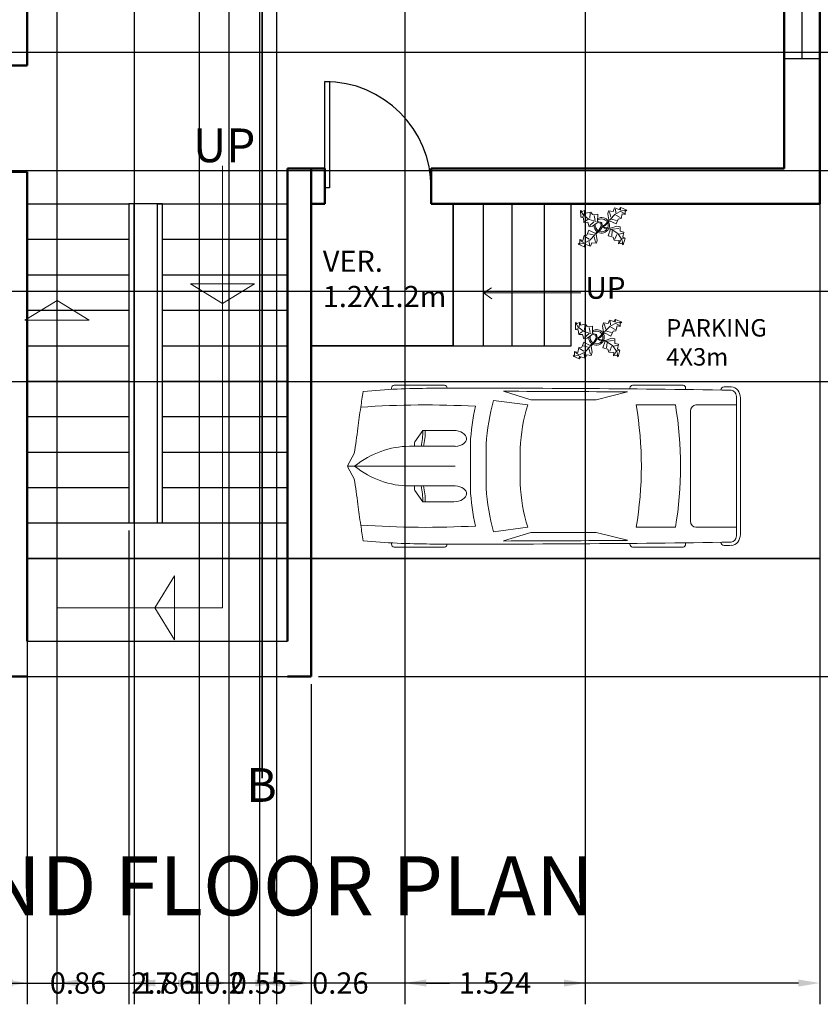
# Model space of a CAD drawing. Units: metres. Extents: x 2443.7 to 2482.9, y 2261.4 to 2287.
# Tile 2 of 8: x 2451.1 to 2457.9, y 2261.4 to 2269.7. Entities that reach past the tile are written whole.
import ezdxf

# ---------------------------------------------------------------- set-up
doc = ezdxf.new("R2010")
doc.units = ezdxf.units.M
doc.linetypes.add('ACAD_ISO02W100', pattern=[15, 12, -3])
for name, color, linetype, lineweight in [('A-ANNO-DIMS', 2, 'Continuous', 18), ('A-ANNO-SYMB', 1, 'Continuous', 18), ('A-AREA-IDEN', 11, 'Continuous', 25), ('A-FLOR-PROJ', 7, 'ACAD_ISO02W100', 18), ('A-MODL', 7, 'Continuous', 25), ('A-WALL', 7, 'Continuous', 50), ('car', 150, 'Continuous', 18), ('door', 6, 'Continuous', 25), ('floor', 7, 'Continuous', 35), ('flower', 70, 'Continuous', 18), ('section', 1, 'Continuous', 35), ('stair', 2, 'Continuous', 25), ('text', 11, 'Continuous', 25), ('window', 3, 'Continuous', 25)]:
    doc.layers.add(name, color=color, linetype=linetype, lineweight=lineweight)
doc.styles.get("Standard").update_dxf_attribs({"font": 'arial.ttf'})
doc.dimstyles.get("Standard").update_dxf_attribs({"dimtxt": 0.18, "dimasz": 0.18, "dimexe": 0.18, "dimexo": 0.0625, "dimgap": 0.09, "dimtad": 0, "dimtih": 1, "dimtoh": 1, "dimdec": 4, "dimzin": 0, "dimdsep": 46, "dimtxsty": 'Standard', "dimcen": 0.09, "dimadec": 0, "dimazin": 0, "dimtfac": 1, "dimtdec": 4, "dimtofl": 0, "dimtmove": 0, "dimatfit": 3, "dimfxl": 1, "dimtolj": 1, "dimtzin": 0, "dimarcsym": 0})

# ---------------------------------------------------------------- blocks, each defined once
blk = doc.blocks.new('*U21')
for p, q in [((0, 0), (0, -6)), ((40, 0), (40, -6))]:
    blk.add_line(p, q)
blk.add_lwpolyline([(0, 0), (0, 40), (1.75, 40), (1.75, 0)], close=True)
blk.add_arc((0, 0), 40, 0, 90)
blk = doc.blocks.new('*U2')
for p, q in [((0, 0), (0, -6)), ((-40, 0), (-40, -6))]:
    blk.add_line(p, q)
blk.add_lwpolyline([(0, 0), (0, 40), (-1.75, 40), (-1.75, 0)], close=True)
blk.add_arc((0, 0), 40, 90, 180)
blk = doc.blocks.new('Plant - Rubber or Philodendron')
for p, q in [((-16.2005, 11.4774), (-13.9899, 8.1064)), ((-16.2005, 11.4774), (-14.8639, 10.7964)), ((-16.0159, 6.3329), (-16.2005, 11.4774)), ((-14.8639, 10.7964), (-12.6195, 11.8975)), ((-13.9899, 8.1064), (-9.5434, 4.7185)), ((-13.3174, 8.325), (-13.0735, 11.0065)), ((-12.6195, 11.8975), (-12.1909, 9.4345)), ((-12.1909, 9.4345), (-8.3829, 10.3)), ((-8.8369, 9.409), (-9.0894, 5.6095)), ((-8.3829, 10.3), (-7.0549, 8.501)), ((-7.0549, 8.501), (-3.0284, 8.6941)), ((-4.8529, 4.012), (-5.7184, 7.82)), ((-3.0284, 8.6941), (-3.0709, 3.1041)), ((4.6914, 8.8812), (5.3859, 11.2828)), ((4.6914, 8.8812), (5.5014, 4.4831)), ((5.3859, 11.2828), (8.8871, 10.7908)), ((5.9878, 10.4842), (7.1971, 6.3869)), ((10.3916, 8.7942), (6.2847, 4.4028)), ((8.8871, 10.7908), (9.9809, 13.4933)), ((9.9809, 13.4933), (13.3837, 12.301)), ((15.3859, 11.3055), (10.3916, 8.7942)), ((10.5828, 12.6946), (10.8893, 9.7953)), ((14.2977, 6.1031), (10.9934, 7.9956)), ((13.3837, 12.301), (14.68, 13.9039)), ((14.5816, 13.2037), (14.3848, 11.8033)), ((14.68, 13.9039), (19.3848, 11.8146)), ((15.7909, 9.1065), (14.8995, 5.3044)), ((15.2875, 10.6053), (17.5907, 9.2105)), ((19.3848, 11.8146), (15.3859, 11.3055)), ((18.1925, 8.4119), (15.7909, 9.1065)), ((19.3848, 11.8146), (18.1868, 10.9119)), ((18.1868, 10.9119), (18.1925, 8.4119)), ((-14.0069, 5.8704), (-16.0159, 6.3329)), ((-15.3434, 6.5514), (-13.9984, 6.9884)), ((-13.5868, 2.2894), (-14.0069, 5.8704)), ((-10.6784, 2.491), (-13.5868, 2.2894)), ((-13.1329, 3.1804), (-10.6614, 4.727)), ((-9.5858, -0.8715), (-10.6784, 2.491)), ((-9.5434, 4.7185), (-4.1917, 2.9888)), ((-9.1318, 0.0195), (-5.9793, 2.9025)), ((-7.1228, -0.443), (-3.5248, 2.2131)), ((-3.5248, 2.2131), (-3.3011, 2.4355)), ((-3.3011, 2.4355), (-0.5306, 1.7947)), ((-3.0709, 3.1041), (0.0797, 2.3163)), ((-0.5306, 1.7947), (-0.2255, -0.5527)), ((-0.5306, 1.7947), (-0.5306, 1.7947)), ((0.0797, 2.3163), (0.4866, -0.031)), ((0.4866, -0.031), (2.1141, 0.2298)), ((2.1141, 0.2298), (5.4346, 3.9146)), ((6.1032, 3.6844), (2.8262, -0.031)), ((5.4346, 3.9146), (5.5014, 4.4831)), ((11.1089, 1.1958), (6.1032, 3.6844)), ((7.7005, 4.8881), (11.5025, 3.9967)), ((12.7005, 4.8994), (11.1089, 1.1958)), ((14.8995, 5.3044), (12.7005, 4.8994)), ((-13.5228, -7.6679), (-11.3237, -7.2629)), ((-11.3237, -7.2629), (-9.7321, -3.5593)), ((-6.3237, -7.2516), (-10.1257, -6.3602)), ((-9.7321, -3.5593), (-4.7264, -6.0479)), ((-7.1228, -0.443), (-9.5858, -0.8715)), ((-9.0148, -11.1577), (-4.9047, -6.8122)), ((-2.019, -3.6148), (-4.7264, -6.0479)), ((-4.1246, -6.8466), (-4.0579, -6.2781)), ((-3.3146, -11.2447), (-4.1246, -6.8466)), ((-4.0579, -6.2781), (-0.9375, -3.1608)), ((-2.019, -3.6148), (-0.2255, -0.5527)), ((-0.9375, -3.1608), (0.5883, -0.8135)), ((0.5883, -0.8135), (2.2447, -2.0916)), ((2.8262, -0.031), (1.3003, -0.5527)), ((1.3003, -0.5527), (2.4193, -1.4655)), ((2.2447, -2.0916), (6.7108, -2.6626)), ((2.4193, -1.4655), (6.895, -2.1175)), ((4.943, -7.9659), (6.7108, -2.6626)), ((11.6605, -0.5413), (6.895, -2.1175)), ((12.3677, -6.1981), (7.219, -2.6772)), ((8.125, -4.0768), (7.7715, -7.9659)), ((8.3544, -2.7453), (13.1973, -2.1704)), ((10.2463, -10.4408), (11.6605, -6.9053)), ((11.6605, -0.5413), (14.1354, -0.8948)), ((15.5496, -10.7943), (12.3677, -6.1981)), ((16.2567, -5.8446), (13.4283, -6.5517)), ((14.1354, -0.8948), (14.1354, -4.4304)), ((14.1354, -4.4304), (16.9638, -5.1375)), ((16.9638, -5.1375), (16.2567, -8.673)), ((-18.008, -14.1781), (-16.8101, -13.2754)), ((-18.008, -14.1781), (-14.0091, -13.669)), ((-13.3032, -16.2674), (-18.008, -14.1781)), ((-16.8157, -10.7754), (-14.4141, -11.4699)), ((-16.8101, -13.2754), (-16.8157, -10.7754)), ((-13.9107, -12.9688), (-16.2139, -11.574)), ((-14.4141, -11.4699), (-13.5228, -7.6679)), ((-14.0091, -13.669), (-9.0148, -11.1577)), ((-12.0069, -14.6645), (-13.3032, -16.2674)), ((-13.2048, -15.5672), (-13.008, -14.1668)), ((-12.921, -8.4665), (-9.6166, -10.359)), ((-8.6042, -15.8568), (-12.0069, -14.6645)), ((-9.206, -15.0581), (-9.5126, -12.1588)), ((-7.5103, -13.1543), (-8.6042, -15.8568)), ((-4.0092, -13.6463), (-7.5103, -13.1543)), ((-4.611, -12.8477), (-5.8203, -8.7504)), ((-3.3146, -11.2447), (-4.0092, -13.6463)), ((8.8321, -9.0266), (4.943, -7.9659)), ((9.5392, -11.1479), (8.8321, -9.0266)), ((13.4283, -11.5015), (9.5392, -11.1479)), ((13.0748, -13.9763), (13.4283, -11.5015)), ((15.5496, -13.6228), (13.0748, -13.9763)), ((14.8425, -10.7943), (13.7819, -13.2692)), ((16.6103, -14.6834), (15.5496, -10.7943)), ((16.6103, -14.6834), (15.5496, -13.6228)), ((17.3174, -9.7337), (15.9032, -9.7337)), ((16.2567, -8.673), (18.0245, -9.7337)), ((18.0245, -9.7337), (16.6103, -14.6834))]:
    blk.add_line(p, q)
for centre, radius, start, end in [((0.0308, 0.1664), 6, 178.6147, 235.1169), ((0.0308, 0.1664), 5, 168.1647, 238.6725), ((0, 0), 6.1275, 34.37569, 120.1028), ((-0.0601, -0.2075), 5.2461, 33.82192, 124.9414), ((-0.2664, 0.1682), 5.2775, 338.4094, 20.03007), ((-0.098, 0.1364), 6.1288, 341.2017, 26.09184), ((-0.0234, 0.3825), 6.1492, 242.5812, 331.2714), ((-0.1102, 0.4886), 5.2883, 247.3711, 327.472)]:
    blk.add_arc(centre, radius, start, end)
blk = doc.blocks.new('*U17')
for p, q in [((46.55, 38.89), (22.35, 38.89)), ((136.7, 38.89), (160.9, 38.89)), ((21.1, 37.41), (21.1, 36.83)), ((47.8, 37.39), (47.8, 37.41)), ((87.99, 31.87), (74.76, 35.92)), ((134.31, 35.6), (119.29, 31.78)), ((135.45, 37.07), (135.45, 37.41)), ((162.15, 37.41), (162.15, 36.77)), ((186.47, -33.5), (186.47, 33.5)), ((70.03, 31.54), (86.41, 29.35)), ((138.42, 29.35), (157.25, 29.35)), ((186.47, 29.35), (167.01, 29.35)), ((188.4, -32.76), (188.4, 32.76)), ((164.52, 26.39), (164.52, -26.39)), ((32.27, 11.63), (36.13, 17.17)), ((36.13, 17.17), (50.94, 17.17)), ((29.77, 9.51), (51.68, 9.51)), ((32.12, 9.51), (32.12, 11.15)), ((58.92, -10.77), (58.92, 10.77)), ((66.55, -10.53), (66.55, 10.53)), ((186.47, -10.53), (186.47, 10.53)), ((3.27, 6.13), (0.1, 0.41)), ((82.74, 8.5), (82.74, -8.5)), ((0, 0), (51.68, 0)), ((0.1, -0.41), (3.27, -6.13)), ((29.77, -9.51), (51.68, -9.51)), ((32.12, -9.51), (32.12, -11.15)), ((32.27, -11.63), (36.13, -17.17)), ((36.13, -17.17), (50.94, -17.17)), ((86.41, -29.35), (70.03, -31.54)), ((87.99, -31.87), (74.76, -35.92)), ((134.31, -35.6), (119.29, -31.78)), ((157.25, -29.35), (138.42, -29.35)), ((167.01, -29.35), (186.47, -29.35)), ((21.1, -37.41), (21.1, -36.83)), ((47.8, -37.39), (47.8, -37.41)), ((135.45, -37.07), (135.45, -37.41)), ((162.15, -37.41), (162.15, -36.77)), ((46.55, -38.89), (22.35, -38.89)), ((136.7, -38.89), (160.9, -38.89))]:
    blk.add_line(p, q)
for centre, major_axis, ratio, start_param, end_param in [((22.35, 37.41), (0, -1.48), 0.842304, 3.141593, 4.712389), ((46.55, 37.41), (0, 1.48), 0.842304, -1.570796, 0), ((136.7, 37.41), (0, -1.48), 0.842304, 3.141593, 4.712389), ((160.9, 37.41), (0, 1.48), 0.842304, -1.570796, 0), ((180.63, 35.84), (0, 2.22), 0.842304, -0.013017, 1.249894), ((64.48, -10556.36), (0, 10595.31), 0.842304, -0.013397, -0.013017), ((183.98, 32.76), (0, -5.25), 0.842304, 1.570796, 3.128196), ((266.03, -27.52), (0, 313.31), 0.842304, 1.367076, 1.39176), ((41.19, -490.86), (0, 528.23), 0.842304, 0.00281, 0.075598), ((64.48, -10555.62), (0, 10593.03), 0.842304, -0.013397, 0.002797), ((64.48, -10555.62), (0, -10591.55), 0.842304, 3.133765, 3.140441), ((183.98, 33.5), (0, -2.96), 0.842304, 1.570796, 3.128196), ((37.47, -593.96), (0, -623.33), 0.842304, 3.096046, 3.200911), ((134.4, 5.39), (0, -89.78), 0.842304, 4.449482, 4.652344), ((135.29, 5.39), (0, 81.77), 0.842304, 1.245306, 1.50788), ((149.6, 2.8), (0, -79.58), 0.842304, 4.372215, 4.640744), ((95.79, -3666.35), (0, -3698.24), 0.842304, 3.134049, 3.144098), ((17.08, 0), (0, 147.02), 0.842304, 4.511394, 4.913384), ((35.91, 0), (0, 147.02), 0.842304, 4.511394, 4.913384), ((167.01, 26.39), (0, 2.96), 0.842304, 0, 1.570796), ((259.18, -27.52), (0, -305.3), 0.842304, 4.528606, 4.561838), ((-204.49, 52.4), (0, -250.96), 0.842304, 1.385369, 1.434372), ((13.04, 17.01), (0, 27.42), 0.842304, 4.435146, 4.718221), ((14.2, 17.01), (0, 27.42), 0.842304, 4.435146, 4.718221), ((50.79, 13.34), (6.34, -0.36), 0.603834, -1.395552, 1.581315), ((29.77, -46.66), (0, 56.17), 0.842304, 0, 0.590319), ((32.75, 11.15), (0, 0.74), 0.842304, 0.879714, 1.570796), ((0.62, 0), (0, -0.74), 0.842304, 4.131459, 5.293319), ((29.77, 46.66), (0, 56.17), 0.842304, 2.551274, 3.141593), ((-204.49, -52.4), (0, 250.96), 0.842304, -1.434372, -1.385369), ((149.6, -2.8), (0, -79.58), 0.842304, -1.499151, -1.230623), ((32.75, -11.15), (0, -0.74), 0.842304, 4.712389, 5.403472), ((13.04, -17.01), (0, -27.42), 0.842304, 1.564964, 1.848039), ((14.2, -17.01), (0, -27.42), 0.842304, 1.564964, 1.848039), ((134.4, -5.39), (0, -89.78), 0.842304, -1.510751, -1.307889), ((135.29, -5.39), (0, -81.77), 0.842304, -1.50788, -1.245306), ((259.18, 27.52), (0, 305.3), 0.842304, 1.721348, 1.754579), ((266.03, 27.52), (0, 313.31), 0.842304, 1.749832, 1.774517), ((37.47, 593.96), (0, -623.33), 0.842304, -0.059319, 0.045547), ((167.01, -26.39), (0, -2.96), 0.842304, 4.712389, 6.283185), ((95.79, 3666.35), (0, -3698.24), 0.842304, -0.002505, 0.007544), ((183.98, -32.76), (0, -5.25), 0.842304, 0.013397, 1.570796), ((41.19, 490.86), (0, -528.23), 0.842304, -0.075598, -0.00281), ((22.35, -37.41), (0, 1.48), 0.842304, 1.570796, 3.141593), ((64.48, 10555.62), (0, 10593.03), 0.842304, 3.138796, 3.15499), ((46.55, -37.41), (0, -1.48), 0.842304, 0, 1.570796), ((64.48, 10555.62), (0, -10591.55), 0.842304, 0.001152, 0.007828), ((136.7, -37.41), (0, -1.48), 0.842304, -1.570796, 0), ((160.9, -37.41), (0, 1.48), 0.842304, 3.141593, 4.712389), ((180.63, -35.84), (0, -2.22), 0.842304, -1.249894, 0.013017), ((183.98, -33.5), (0, 2.96), 0.842304, 3.15499, 4.712389), ((64.48, 10556.36), (0, 10595.31), 0.842304, 3.15461, 3.15499)]:
    blk.add_ellipse(centre, major_axis=major_axis, ratio=ratio, start_param=start_param, end_param=end_param)
at = {"extrusion": (0, 0, -1)}
blk.add_ellipse((50.79, -13.34), major_axis=(6.34, 0.36), ratio=0.603834, start_param=-1.395552, end_param=1.581315, dxfattribs=at)
blk = doc.blocks.new('aditya')
at = {"layer": 'A-ANNO-SYMB'}
for p, q in [((5.15, 3.6226), (5.15, -0.1171)), ((3.752, -0.1171), (3.752, 3.3)), ((5.4209, 2.6227), (4.8791, 2.6227)), ((4.8791, 2.6227), (5.15, 2.4567)), ((5.4209, 2.6227), (5.15, 2.4567)), ((7.3585, 2.5465), (7.4248, 2.5908)), ((8.1818, 2.5465), (7.3585, 2.5465)), ((7.3585, 2.5465), (7.4267, 2.4975)), ((3.481, 2.316), (3.752, 2.4819)), ((4.0229, 2.316), (3.752, 2.4819)), ((3.481, 2.316), (4.0229, 2.316)), ((4.7446, 0.1538), (4.5786, -0.1171)), ((4.7446, -0.388), (4.7446, 0.1538)), ((5.15, -0.1171), (3.752, -0.1171)), ((4.7446, -0.388), (4.5786, -0.1171))]:
    blk.add_line(p, q, dxfattribs=at)
at = {"layer": 'A-FLOR-PROJ', "ltscale": 0.01}
blk.add_line((10.2, 3.3), (10.2, 0.3), dxfattribs=at)
at = {"layer": 'A-WALL'}
for p, q in [((10.2, 3.3), (10.2, 9.9)), ((3.5, 4.4718), (3.5, 5.1521)), ((9.9, 4.8), (9.9, 5)), ((9.9, 3.6), (9.9, 4.8)), ((5.7, -0.4), (5.7, 3.6)), ((5.9, 3.6), (5.7, 3.6)), ((5.9, -0.7), (5.9, 3.6)), ((5.9, 3.6), (6.0153, 3.6)), ((6.9153, 3.6), (9.9, 3.6)), ((3.5, -0.4), (3.5, 3.5718)), ((5.9, 3.3), (6.0153, 3.3)), ((6.9153, 3.3), (10.2, 3.3)), ((3.5, -0.7), (3.2, -0.7)), ((5.7, -0.7), (5.9, -0.7))]:
    blk.add_line(p, q, dxfattribs=at)
for points in [[(3.3, 4.4718), (3.5, 4.4718)], [(6.0153, 3.3), (6.0153, 3.6)], [(6.9153, 3.6), (6.9153, 3.3)], [(3.5, 3.5718), (3.3, 3.5718), (3.3, 3.5742)]]:
    blk.add_lwpolyline(points, dxfattribs=at)
at = {"layer": 'floor'}
for p, q in [((3.5, 0.3), (5.7, 0.3)), ((5.7, 0.3), (9.9, 0.3)), ((10.2, 0.3), (9.9, 0.3))]:
    blk.add_line(p, q, dxfattribs=at)
blk.add_lwpolyline([(6.9153, 3.3), (7.1, 3.3), (7.1, 2.1), (5.9, 2.1), (5.9, 3.3), (6.0153, 3.3)], dxfattribs=at)
at = {"layer": 'section'}
blk.add_line((5.4866, -1.5581), (5.4866, 11.3875), dxfattribs=at)
at = {"layer": 'stair'}
for p, q in [((3.5, 3.3), (4.3595, 3.3)), ((4.6, 3.3), (5.7, 3.3)), ((7.3585, 2.1), (7.3585, 3.3)), ((7.6, 2.1), (7.6, 3.3)), ((7.873, 2.1), (7.873, 3.3)), ((8.1, 2.1), (8.1, 3.3)), ((3.5, 3), (4.3595, 3)), ((4.6423, 3), (5.7, 3)), ((3.5, 2.7), (4.3595, 2.7)), ((4.6423, 2.7), (5.7, 2.7)), ((3.5, 2.4), (4.3595, 2.4)), ((4.6423, 2.4), (5.7, 2.4)), ((3.5, 2.1), (4.3595, 2.1)), ((4.6423, 2.1), (5.7, 2.1)), ((7.1, 2.1), (8.1, 2.1)), ((3.5, 1.8), (4.3595, 1.8)), ((4.6423, 1.8), (5.7, 1.8)), ((3.5, 1.5), (4.3595, 1.5)), ((4.6423, 1.5), (5.7, 1.5)), ((3.5, 1.2), (4.3595, 1.2)), ((4.6423, 1.2), (5.7, 1.2)), ((3.5, 0.9), (4.3595, 0.9)), ((4.6423, 0.9), (5.7, 0.9)), ((3.5, 0.6), (5.7, 0.6)), ((3.5, 0.3), (5.7, 0.3)), ((3.5, -0.4), (5.7, -0.4)), ((3.5, -0.7), (5.7, -0.7))]:
    blk.add_line(p, q, dxfattribs=at)
for points in [[(4.6423, 3.3002), (4.3595, 3.3002), (4.3595, 0.6), (4.6423, 0.6)], [(4.6008, 3.3002), (4.4009, 3.3002), (4.4001, 0.6), (4.6, 0.6)]]:
    blk.add_lwpolyline(points, close=True, dxfattribs=at)
at = {"layer": 'window'}
blk.add_line((10.05, 5.7272), (10.05, 4.5272), dxfattribs=at)
blk.add_lwpolyline([(9.9, 5.7272), (10.2, 5.7272), (10.2, 4.5272), (9.9, 4.5272)], close=True, dxfattribs=at)
at = {"layer": 'car', "xscale": 0.0176302179033872, "yscale": 0.0176302179033872, "zscale": 0.0176302179033872}
blk.add_blockref('*U17', (6.2077, 1.081), dxfattribs=at)
at = {"layer": 'door', "xscale": 0.0224999999999983, "yscale": 0.0224999999999983, "zscale": 0.0224999999999983, "rotation": 90}
blk.add_blockref('*U2', (3.365, 4.4718), dxfattribs=at)
at = {"layer": 'door', "xscale": 0.0224999999999983, "yscale": 0.0224999999999983, "zscale": 0.0224999999999983}
blk.add_blockref('*U21', (6.0153, 3.435), dxfattribs=at)
at = {"layer": 'flower', "xscale": 0.0110121980909997, "yscale": 0.0110121980909997, "zscale": 0.0110121980909997}
for p in [(8.3562, 3.1165), (8.3127, 2.1687)]:
    blk.add_blockref('Plant - Rubber or Philodendron', p, dxfattribs=at)
at = {"layer": 'A-AREA-IDEN', "attachment_point": 1}
for s, width, gutter_width, insert, char_height in [('{\\fArial|b1|i1|c0|p34;VER.\\P1.2X1.2m}', 7.547056, 5.5992, (5.9989, 2.9045), 0.179173), ('{\\fArial|b1|i1|c0|p34;PARKING\\P4X3m}', 6.208347, 4.606, (8.9024, 2.3248), 0.147391)]:
    blk.add_mtext_dynamic_manual_height_columns(s, width=width, gutter_width=gutter_width, heights=[0], dxfattribs=dict(at, insert=insert, char_height=char_height))
at = {"layer": 'text'}
for s, height, p in [('UP', 0.28528, (4.9018, 3.6525)), ('UP', 0.18457, (8.2182, 2.4969)), ('B', 0.2853, (5.3539, -1.7595))]:
    blk.add_text(s, height=height, dxfattribs=at).set_placement(p)
at = {"layer": 'text', "insert": (1.2226, -2.2194), "char_height": 0.5, "attachment_point": 1}
blk.add_mtext_dynamic_manual_height_columns('{\\fArial|b1|i1|c0|p34;GROUND FLOOR PLAN}', width=17.015787, gutter_width=7.8414, heights=[0], dxfattribs=at)
blk = doc.blocks.new('*D22')
at = {"layer": 'A-ANNO-DIMS', "color": 0, "lineweight": -2, "transparency": 16777216}
for p, q in [((2457.8828, 2265.0972), (2457.8828, 2261.3876)), ((2447.6828, 2264.7972), (2447.6828, 2261.3876)), ((2447.8628, 2261.5676), (2452.4684, 2261.5676)), ((2457.7028, 2261.5676), (2453.0971, 2261.5676))]:
    blk.add_line(p, q, dxfattribs=at)
at = {"layer": 'A-ANNO-DIMS', "color": 0, "transparency": 16777216}
for points in [[(2447.8628, 2261.5976), (2447.8628, 2261.5376), (2447.6828, 2261.5676)], [(2457.7028, 2261.5976), (2457.7028, 2261.5376), (2457.8828, 2261.5676)]]:
    blk.add_solid(points, dxfattribs=at)
at = {"layer": 'Defpoints', "color": 0, "transparency": 16777216}
for p in [(2457.8828, 2265.1597), (2447.6828, 2264.8597), (2457.8828, 2261.5676)]:
    blk.add_point(p, dxfattribs=at)
at = {"layer": 'A-ANNO-DIMS', "color": 0, "transparency": 16777216, "insert": (2452.7828, 2261.5676), "char_height": 0.18, "attachment_point": 5}
blk.add_mtext('\\A1;10.2', dxfattribs=at)
blk = doc.blocks.new('*D23')
at = {"layer": 'A-ANNO-DIMS', "color": 0, "lineweight": -2, "transparency": 16777216}
for p, q in [((2457.9453, 2274.7597), (2482.2428, 2274.7597)), ((2482.0628, 2274.5797), (2482.0628, 2269.6416)), ((2482.0628, 2264.3397), (2482.0628, 2269.2778)), ((2453.6453, 2264.1597), (2482.2428, 2264.1597))]:
    blk.add_line(p, q, dxfattribs=at)
at = {"layer": 'A-ANNO-DIMS', "color": 0, "transparency": 16777216}
for points in [[(2482.0328, 2274.5797), (2482.0928, 2274.5797), (2482.0628, 2274.7597)], [(2482.0328, 2264.3397), (2482.0928, 2264.3397), (2482.0628, 2264.1597)]]:
    blk.add_solid(points, dxfattribs=at)
at = {"layer": 'Defpoints', "color": 0, "transparency": 16777216}
for p in [(2457.8828, 2274.7597), (2453.5828, 2264.1597), (2482.0628, 2264.1597)]:
    blk.add_point(p, dxfattribs=at)
at = {"layer": 'A-ANNO-DIMS', "color": 0, "transparency": 16777216, "insert": (2482.0628, 2269.4597), "char_height": 0.18, "attachment_point": 5}
blk.add_mtext('\\A1;10.6', dxfattribs=at)
blk = doc.blocks.new('*D25')
at = {"layer": 'A-ANNO-DIMS', "color": 0, "lineweight": -2, "transparency": 16777216}
for p, q in [((2450.8828, 2264.0972), (2450.8828, 2261.3876)), ((2453.5828, 2264.0972), (2453.5828, 2261.3876)), ((2451.0628, 2261.5676), (2451.9774, 2261.5676)), ((2453.4028, 2261.5676), (2452.4882, 2261.5676))]:
    blk.add_line(p, q, dxfattribs=at)
at = {"layer": 'A-ANNO-DIMS', "color": 0, "transparency": 16777216}
for points in [[(2451.0628, 2261.5976), (2451.0628, 2261.5376), (2450.8828, 2261.5676)], [(2453.4028, 2261.5976), (2453.4028, 2261.5376), (2453.5828, 2261.5676)]]:
    blk.add_solid(points, dxfattribs=at)
at = {"layer": 'Defpoints', "color": 0, "transparency": 16777216}
for p in [(2450.8828, 2264.1597), (2453.5828, 2264.1597), (2453.5828, 2261.5676)]:
    blk.add_point(p, dxfattribs=at)
at = {"layer": 'A-ANNO-DIMS', "color": 0, "transparency": 16777216, "insert": (2452.2328, 2261.5676), "char_height": 0.18, "attachment_point": 5}
blk.add_mtext('\\A1;2.7', dxfattribs=at)
blk = doc.blocks.new('*D38')
at = {"layer": 'A-ANNO-DIMS', "color": 0, "lineweight": -2, "transparency": 16777216}
for p, q in [((2454.3757, 2273.1253), (2454.3757, 2261.3876)), ((2455.8997, 2273.1253), (2455.8997, 2261.3876)), ((2454.5557, 2261.5676), (2454.7528, 2261.5676)), ((2455.7197, 2261.5676), (2455.5225, 2261.5676))]:
    blk.add_line(p, q, dxfattribs=at)
at = {"layer": 'A-ANNO-DIMS', "color": 0, "transparency": 16777216}
for points in [[(2454.5557, 2261.5976), (2454.5557, 2261.5376), (2454.3757, 2261.5676)], [(2455.7197, 2261.5976), (2455.7197, 2261.5376), (2455.8997, 2261.5676)]]:
    blk.add_solid(points, dxfattribs=at)
at = {"layer": 'Defpoints', "color": 0, "transparency": 16777216}
for p in [(2454.3757, 2273.1878), (2455.8997, 2273.1878), (2454.3757, 2261.5676)]:
    blk.add_point(p, dxfattribs=at)
at = {"layer": 'A-ANNO-DIMS', "color": 0, "transparency": 16777216, "insert": (2455.1377, 2261.5676), "char_height": 0.18, "attachment_point": 5}
blk.add_mtext('\\A1;1.524', dxfattribs=at)
blk = doc.blocks.new('*D44')
at = {"layer": 'A-ANNO-DIMS', "color": 0, "lineweight": -2, "transparency": 16777216}
for p, q in [((2452.0859, 2270), (2452.0859, 2261.3876)), ((2452.6364, 2270), (2452.6364, 2261.3876)), ((2452.2659, 2261.5676), (2452.4564, 2261.5676)), ((2452.6364, 2261.5676), (2452.8164, 2261.5676))]:
    blk.add_line(p, q, dxfattribs=at)
at = {"layer": 'A-ANNO-DIMS', "color": 0, "transparency": 16777216}
for points in [[(2452.2659, 2261.5976), (2452.2659, 2261.5376), (2452.0859, 2261.5676)], [(2452.4564, 2261.5976), (2452.4564, 2261.5376), (2452.6364, 2261.5676)]]:
    blk.add_solid(points, dxfattribs=at)
at = {"layer": 'Defpoints', "color": 0, "transparency": 16777216}
for p in [(2452.0859, 2270.0625), (2452.6364, 2270.0625), (2452.6364, 2261.5676)]:
    blk.add_point(p, dxfattribs=at)
at = {"layer": 'A-ANNO-DIMS', "color": 0, "transparency": 16777216, "insert": (2453.1409, 2261.5676), "char_height": 0.18, "attachment_point": 5}
blk.add_mtext('\\A1;0.55', dxfattribs=at)
blk = doc.blocks.new('*D47')
at = {"layer": 'A-ANNO-DIMS', "color": 0, "lineweight": -2, "transparency": 16777216}
for p, q in [((2482.0628, 2267.4197), (2482.0628, 2267.5997)), ((2482.0628, 2267.5997), (2482.2428, 2267.5997)), ((2448.9684, 2267.4197), (2482.2428, 2267.4197)), ((2482.0628, 2266.8377), (2482.0628, 2267.2397)), ((2448.9684, 2266.6577), (2482.2428, 2266.6577))]:
    blk.add_line(p, q, dxfattribs=at)
at = {"layer": 'A-ANNO-DIMS', "color": 0, "transparency": 16777216}
for points in [[(2482.0328, 2267.2397), (2482.0928, 2267.2397), (2482.0628, 2267.4197)], [(2482.0328, 2266.8377), (2482.0928, 2266.8377), (2482.0628, 2266.6577)]]:
    blk.add_solid(points, dxfattribs=at)
at = {"layer": 'Defpoints', "color": 0, "transparency": 16777216}
for p in [(2448.9059, 2267.4197), (2482.0628, 2267.4197), (2448.9059, 2266.6577)]:
    blk.add_point(p, dxfattribs=at)
at = {"layer": 'A-ANNO-DIMS', "color": 0, "transparency": 16777216, "insert": (2482.6356, 2267.5997), "char_height": 0.18, "attachment_point": 5}
blk.add_mtext('\\A1;0.762', dxfattribs=at)
blk = doc.blocks.new('*D49')
at = {"layer": 'A-ANNO-DIMS', "color": 0, "lineweight": -2, "transparency": 16777216}
for p, q in [((2448.3865, 2269.4443), (2482.2428, 2269.4443)), ((2482.0628, 2269.2643), (2482.0628, 2269.1253)), ((2482.0628, 2268.6224), (2482.0628, 2268.7615)), ((2448.3865, 2268.4424), (2482.2428, 2268.4424))]:
    blk.add_line(p, q, dxfattribs=at)
at = {"layer": 'A-ANNO-DIMS', "color": 0, "transparency": 16777216}
for points in [[(2482.0328, 2269.2643), (2482.0928, 2269.2643), (2482.0628, 2269.4443)], [(2482.0328, 2268.6224), (2482.0928, 2268.6224), (2482.0628, 2268.4424)]]:
    blk.add_solid(points, dxfattribs=at)
at = {"layer": 'Defpoints', "color": 0, "transparency": 16777216}
for p in [(2448.324, 2269.4443), (2482.0628, 2269.4443), (2448.324, 2268.4424)]:
    blk.add_point(p, dxfattribs=at)
at = {"layer": 'A-ANNO-DIMS', "color": 0, "transparency": 16777216, "insert": (2482.0628, 2268.9434), "char_height": 0.18, "attachment_point": 5}
blk.add_mtext('\\A1;1.00', dxfattribs=at)
blk = doc.blocks.new('*D52')
at = {"layer": 'A-ANNO-DIMS', "color": 0, "lineweight": -2, "transparency": 16777216}
for p, q in [((2451.182762, 2265.397173), (2451.182762, 2261.387605)), ((2452.042262, 2265.397173), (2452.042262, 2261.387605)), ((2451.002762, 2261.567605), (2450.822762, 2261.567605)), ((2452.222262, 2261.567605), (2452.402262, 2261.567605))]:
    blk.add_line(p, q, dxfattribs=at)
at = {"layer": 'A-ANNO-DIMS', "color": 0, "transparency": 16777216}
for points in [[(2451.002762, 2261.597605), (2451.002762, 2261.537605), (2451.182762, 2261.567605)], [(2452.222262, 2261.597605), (2452.222262, 2261.537605), (2452.042262, 2261.567605)]]:
    blk.add_solid(points, dxfattribs=at)
at = {"layer": 'Defpoints', "color": 0, "transparency": 16777216}
for p in [(2451.182762, 2265.459673), (2452.042262, 2265.459673), (2452.042262, 2261.567605)]:
    blk.add_point(p, dxfattribs=at)
at = {"layer": 'A-ANNO-DIMS', "color": 0, "transparency": 16777216, "insert": (2451.612512, 2261.567605), "char_height": 0.18, "attachment_point": 5}
blk.add_mtext('\\A1;0.86', dxfattribs=at)
blk = doc.blocks.new('*D55')
at = {"layer": 'A-ANNO-DIMS', "color": 0, "lineweight": -2, "transparency": 16777216}
for p, q in [((2452.8879, 2274.2987), (2452.8879, 2261.3876)), ((2453.1465, 2274.2987), (2453.1465, 2261.3876)), ((2452.7079, 2261.5676), (2452.5279, 2261.5676)), ((2453.3265, 2261.5676), (2453.5065, 2261.5676))]:
    blk.add_line(p, q, dxfattribs=at)
at = {"layer": 'A-ANNO-DIMS', "color": 0, "transparency": 16777216}
for points in [[(2452.7079, 2261.5976), (2452.7079, 2261.5376), (2452.8879, 2261.5676)], [(2453.3265, 2261.5976), (2453.3265, 2261.5376), (2453.1465, 2261.5676)]]:
    blk.add_solid(points, dxfattribs=at)
at = {"layer": 'Defpoints', "color": 0, "transparency": 16777216}
for p in [(2452.8879, 2274.3612), (2453.1465, 2274.3612), (2453.1465, 2261.5676)]:
    blk.add_point(p, dxfattribs=at)
at = {"layer": 'A-ANNO-DIMS', "color": 0, "transparency": 16777216, "insert": (2453.8302, 2261.5676), "char_height": 0.18, "attachment_point": 5}
blk.add_mtext('\\A1;0.26', dxfattribs=at)
blk = doc.blocks.new('*D63')
at = {"layer": 'A-ANNO-DIMS', "color": 0, "lineweight": -2, "transparency": 16777216}
for p, q in [((2447.6828, 2278.9987), (2447.6828, 2261.3876)), ((2457.8828, 2278.9987), (2457.8828, 2261.3876)), ((2447.8628, 2261.5676), (2452.4684, 2261.5676)), ((2457.7028, 2261.5676), (2453.0971, 2261.5676))]:
    blk.add_line(p, q, dxfattribs=at)
at = {"layer": 'A-ANNO-DIMS', "color": 0, "transparency": 16777216}
for points in [[(2447.8628, 2261.5976), (2447.8628, 2261.5376), (2447.6828, 2261.5676)], [(2457.7028, 2261.5976), (2457.7028, 2261.5376), (2457.8828, 2261.5676)]]:
    blk.add_solid(points, dxfattribs=at)
at = {"layer": 'Defpoints', "color": 0, "transparency": 16777216}
for p in [(2447.6828, 2279.0612), (2457.8828, 2279.0612), (2457.8828, 2261.5676)]:
    blk.add_point(p, dxfattribs=at)
at = {"layer": 'A-ANNO-DIMS', "color": 0, "transparency": 16777216, "insert": (2452.7828, 2261.5676), "char_height": 0.18, "attachment_point": 5}
blk.add_mtext('\\A1;10.2', dxfattribs=at)
blk = doc.blocks.new('*D71')
at = {"layer": 'A-ANNO-DIMS', "color": 0, "lineweight": -2, "transparency": 16777216}
for p, q in [((2451.4341, 2281.6186), (2451.4341, 2261.3876)), ((2453.2904, 2281.6186), (2453.2904, 2261.3876)), ((2451.6141, 2261.5676), (2452.047, 2261.5676)), ((2453.1104, 2261.5676), (2452.6775, 2261.5676))]:
    blk.add_line(p, q, dxfattribs=at)
at = {"layer": 'A-ANNO-DIMS', "color": 0, "transparency": 16777216}
for points in [[(2451.6141, 2261.5976), (2451.6141, 2261.5376), (2451.4341, 2261.5676)], [(2453.1104, 2261.5976), (2453.1104, 2261.5376), (2453.2904, 2261.5676)]]:
    blk.add_solid(points, dxfattribs=at)
at = {"layer": 'Defpoints', "color": 0, "transparency": 16777216}
for p in [(2451.4341, 2281.6811), (2453.2904, 2281.6811), (2453.2904, 2261.5676)]:
    blk.add_point(p, dxfattribs=at)
at = {"layer": 'A-ANNO-DIMS', "color": 0, "transparency": 16777216, "insert": (2452.3623, 2261.5676), "char_height": 0.18, "attachment_point": 5}
blk.add_mtext('\\A1;1.86', dxfattribs=at)

msp = doc.modelspace()

# ---------------------------------------------------------------- block references
at = {"layer": 'A-MODL'}
msp.add_blockref('aditya', (2447.682762, 2264.859673), dxfattribs=at)

# ---------------------------------------------------------------- dimensions: what is measured, and where the dimension line sits
at = {"layer": 'A-ANNO-DIMS'}
for base, p1, p2, override, picture, middle in [((2453.29044, 2261.567605), (2451.43413, 2281.681077), (2453.29044, 2281.681077), {"dimdec": 2, "dimlfac": 1, "dimrnd": 0, "dimzin": 0, "dimdsep": 46, "dimlunit": 2}, '*D71', (2452.362285, 2261.567605)), ((2457.882762, 2261.567605), (2447.682762, 2279.061188), (2457.882762, 2279.061188), {"dimdec": 1, "dimlfac": 1, "dimrnd": 0, "dimzin": 0, "dimdsep": 46, "dimlunit": 2}, '*D63', (2452.782762, 2261.567605)), ((2453.146499, 2261.567605), (2452.887881, 2274.361152), (2453.146499, 2274.361152), {"dimdec": 2, "dimlfac": 1, "dimrnd": 0, "dimzin": 0, "dimdsep": 46, "dimlunit": 2}, '*D55', (2453.830217, 2261.567605)), ((2454.375659, 2261.567605), (2455.89966, 2273.187816), (2454.375659, 2273.187816), {"dimdec": 3, "dimlfac": 1, "dimrnd": 0, "dimzin": 0, "dimdsep": 46, "dimlunit": 2}, '*D38', (2455.13766, 2261.567605)), ((2452.636436, 2261.567605), (2452.085916, 2270.062544), (2452.636436, 2270.062544), {"dimdec": 2, "dimlfac": 1, "dimrnd": 0, "dimzin": 0, "dimdsep": 46, "dimlunit": 2}, '*D44', (2453.14089, 2261.567605)), ((2452.042262, 2261.567605), (2451.182762, 2265.459673), (2452.042262, 2265.459673), {"dimdec": 2, "dimlfac": 1, "dimrnd": 0, "dimzin": 0, "dimdsep": 46, "dimlunit": 2}, '*D52', (2451.612512, 2261.567605)), ((2457.882762, 2261.567605), (2447.682762, 2264.859673), (2457.882762, 2265.159673), {"dimdec": 1, "dimlfac": 1, "dimrnd": 0, "dimzin": 0, "dimdsep": 46, "dimlunit": 2}, '*D22', (2452.782762, 2261.567605)), ((2453.582762, 2261.567605), (2450.882762, 2264.159673), (2453.582762, 2264.159673), {"dimdec": 1, "dimlfac": 1, "dimrnd": 0, "dimzin": 0, "dimdsep": 46, "dimlunit": 2}, '*D25', (2452.232762, 2261.567605))]:
    dim = msp.add_linear_dim(base=base, p1=p1, p2=p2, dimstyle='Standard', override=override, dxfattribs=at)
    dim.commit()
    dim.dimension.update_dxf_attribs({"geometry": picture, "text_midpoint": middle})
for base, p1, p2, override, picture, middle in [((2482.062768, 2264.159673), (2457.882762, 2274.759673), (2453.582762, 2264.159673), {"dimdec": 1, "dimlfac": 1, "dimrnd": 0, "dimzin": 0, "dimdsep": 46, "dimlunit": 2}, '*D23', (2482.062768, 2269.459673)), ((2482.062768, 2269.444297), (2448.323976, 2268.442446), (2448.323976, 2269.444297), {"dimdec": 2, "dimlfac": 1, "dimrnd": 0, "dimzin": 0, "dimdsep": 46, "dimlunit": 2}, '*D49', (2482.062768, 2268.943372)), ((2482.062768, 2267.419676), (2448.905882, 2266.657676), (2448.905882, 2267.419676), {"dimdec": 3, "dimlfac": 1, "dimrnd": 0, "dimzin": 0, "dimdsep": 46, "dimlunit": 2}, '*D47', (2482.635551, 2267.599676))]:
    dim = msp.add_linear_dim(base=base, p1=p1, p2=p2, angle=90, dimstyle='Standard', override=override, dxfattribs=at)
    dim.commit()
    dim.dimension.update_dxf_attribs({"geometry": picture, "text_midpoint": middle})

doc.saveas('drawing.dxf')
